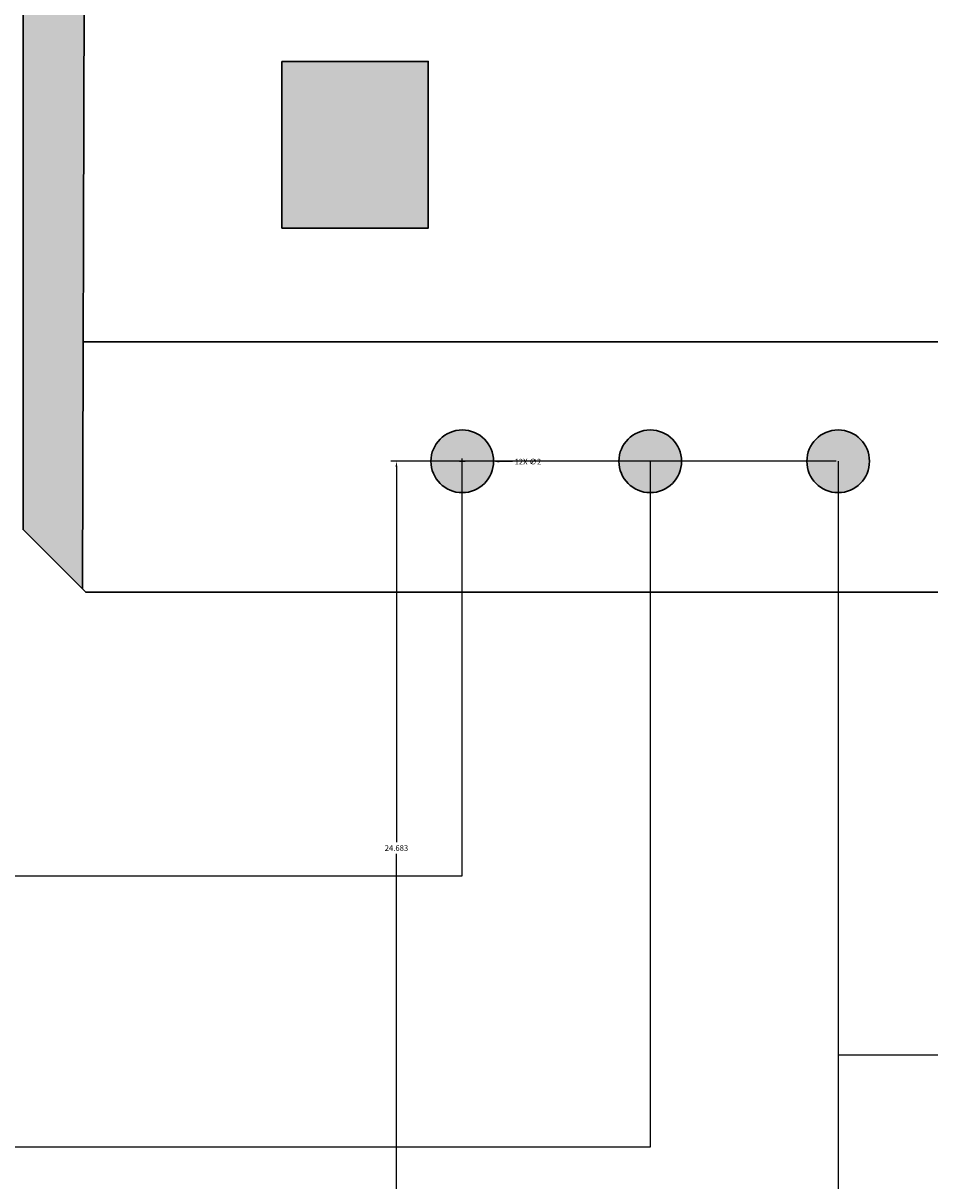
# Model space of a CAD drawing. Units: millimetres. Extents: x -8 to 285, y 5 to 221.
# Tile 5 of 30: x 26 to 55, y 45 to 82. Entities that reach past the tile are written whole.
import ezdxf

# ---------------------------------------------------------------- set-up
doc = ezdxf.new("R2010")
doc.units = ezdxf.units.MM
for name, color, linetype, lineweight in [('A-ANNO-DIMS', 2, 'Continuous', 18), ('E-EQPM-PATT', 252, 'Continuous', 13), ('E-POWR-CTRL', 7, 'Continuous', 30), ('E-POWR-DC-NEG', 3, 'Continuous', 25)]:
    doc.layers.add(name, color=color, linetype=linetype, lineweight=lineweight)
doc.layers.add('E-POWR-DC-POS', color=30, linetype='Continuous', lineweight=25, true_color=0xf26722)
doc.styles.get("Standard").update_dxf_attribs({"font": 'arial.ttf'})
doc.dimstyles.get("Standard").update_dxf_attribs({"dimtxt": 0.18, "dimasz": 0.18, "dimexe": 0.18, "dimexo": 0.0625, "dimgap": 0.09, "dimtad": 0, "dimtih": 1, "dimtoh": 1, "dimdec": 4, "dimzin": 0, "dimdsep": 46, "dimtxsty": 'Standard', "dimcen": 0.09, "dimadec": 0, "dimazin": 0, "dimtfac": 1, "dimtdec": 4, "dimtofl": 0, "dimtmove": 0, "dimatfit": 3, "dimfxl": 1, "dimtolj": 1, "dimtzin": 0, "dimarcsym": 0})

# ---------------------------------------------------------------- blocks, each defined once
blk = doc.blocks.new('*D10')
at = {"layer": 'A-ANNO-DIMS', "color": 0, "lineweight": -2, "transparency": 16777216}
for p, q in [((145.103, 206.457), (-7.608, 206.457)), ((-7.428, 206.277), (-7.428, 113.161)), ((-7.428, 19.682), (-7.428, 112.797)), ((30.453, 19.502), (-7.608, 19.502))]:
    blk.add_line(p, q, dxfattribs=at)
at = {"layer": 'A-ANNO-DIMS', "color": 0, "transparency": 16777216}
for points in [[(-7.458, 206.277), (-7.398, 206.277), (-7.428, 206.457)], [(-7.458, 19.682), (-7.398, 19.682), (-7.428, 19.502)]]:
    blk.add_solid(points, dxfattribs=at)
at = {"layer": 'Defpoints', "color": 0, "transparency": 16777216}
for p in [(-7.428, 206.457), (145.165, 206.457), (30.516, 19.502)]:
    blk.add_point(p, dxfattribs=at)
at = {"layer": 'A-ANNO-DIMS', "color": 0, "transparency": 16777216, "insert": (-7.428, 112.979), "char_height": 0.18, "attachment_point": 5}
blk.add_mtext('\\A1;186.95', dxfattribs=at)
blk = doc.blocks.new('*D21')
at = {"layer": 'A-ANNO-DIMS', "color": 0, "lineweight": -2, "transparency": 16777216}
for p, q in [((52.109, 67.906), (37.892, 67.906)), ((38.072, 67.726), (38.072, 55.747)), ((38.072, 43.404), (38.072, 55.383)), ((52.109, 43.224), (37.892, 43.224))]:
    blk.add_line(p, q, dxfattribs=at)
at = {"layer": 'A-ANNO-DIMS', "color": 0, "transparency": 16777216}
for points in [[(38.042, 67.726), (38.102, 67.726), (38.072, 67.906)], [(38.042, 43.404), (38.102, 43.404), (38.072, 43.224)]]:
    blk.add_solid(points, dxfattribs=at)
at = {"layer": 'Defpoints', "color": 0, "transparency": 16777216}
for p in [(38.072, 67.906), (52.172, 67.906), (52.172, 43.224)]:
    blk.add_point(p, dxfattribs=at)
at = {"layer": 'A-ANNO-DIMS', "color": 0, "transparency": 16777216, "insert": (38.072, 55.565), "char_height": 0.18, "attachment_point": 5}
blk.add_mtext('\\A1;24.683', dxfattribs=at)
blk = doc.blocks.new('*D22')
at = {"layer": 'A-ANNO-DIMS', "color": 0, "lineweight": -2, "transparency": 16777216}
for p, q in [((6.672, 45.959), (6.672, 5.222)), ((30.516, 35.867), (30.516, 5.222)), ((6.852, 5.402), (18.129, 5.402)), ((30.336, 5.402), (19.059, 5.402))]:
    blk.add_line(p, q, dxfattribs=at)
at = {"layer": 'A-ANNO-DIMS', "color": 0, "transparency": 16777216}
for points in [[(6.852, 5.432), (6.852, 5.372), (6.672, 5.402)], [(30.336, 5.432), (30.336, 5.372), (30.516, 5.402)]]:
    blk.add_solid(points, dxfattribs=at)
at = {"layer": 'Defpoints', "color": 0, "transparency": 16777216}
for p in [(6.672, 46.021), (30.516, 35.929), (30.516, 5.402)]:
    blk.add_point(p, dxfattribs=at)
at = {"layer": 'A-ANNO-DIMS', "color": 0, "transparency": 16777216, "insert": (18.594, 5.402), "char_height": 0.18, "attachment_point": 5}
blk.add_mtext('\\A1;23.843', dxfattribs=at)
blk = doc.blocks.new('*D38')
at = {"layer": 'A-ANNO-DIMS', "color": 0, "lineweight": -2, "transparency": 16777216}
for p, q in [((40.172, 67.816), (40.172, 67.996)), ((40.082, 67.906), (40.262, 67.906)), ((41.772, 67.896), (41.352, 67.899))]:
    blk.add_line(p, q, dxfattribs=at)
at = {"layer": 'A-ANNO-DIMS', "color": 0, "transparency": 16777216}
blk.add_solid([(41.352, 67.929), (41.351, 67.869), (41.172, 67.9)], dxfattribs=at)
at = {"layer": 'Defpoints', "color": 0, "transparency": 16777216}
for p in [(39.172, 67.913), (41.172, 67.9)]:
    blk.add_point(p, dxfattribs=at)
at = {"layer": 'A-ANNO-DIMS', "color": 0, "transparency": 16777216, "insert": (42.268, 67.896), "char_height": 0.18, "attachment_point": 5}
blk.add_mtext('\\A1;12X ∅2', dxfattribs=at)

msp = doc.modelspace()

# ---------------------------------------------------------------- hatches: boundary and pattern name
at = {"layer": 'E-EQPM-PATT'}
h = msp.add_hatch(color=256, dxfattribs=at)
h.set_gradient(color2=(0, 0, 0), tint=1)
h.paths.add_polyline_path([(41.1717, 67.9064, 1), (39.1717, 67.9064, 1)])
h.paths.add_polyline_path([(47.1717, 67.9064, 1), (45.1717, 67.9064, 1)])
h.paths.add_polyline_path([(53.1717, 67.9064, 1), (51.1717, 67.9064, 1)])
h.paths.add_polyline_path([(57.1717, 67.9064, 1), (59.1717, 67.9064, 1)])
h.paths.add_polyline_path([(65.1717, 67.9064, 1), (63.1717, 67.9064, 1)])
h.paths.add_polyline_path([(69.1717, 67.9064, 1), (71.1717, 67.9064, 1)])
h.paths.add_polyline_path([(148.1394, 196.6424), (148.1394, 201.7939), (142.1909, 201.7939), (142.1909, 196.6424)])
h.paths.add_polyline_path([(186.1388, 201.7939), (186.1388, 196.6424), (192.0873, 196.6424), (192.0873, 201.7939)])
h.paths.add_polyline_path([(234.0155, 196.6424), (234.0155, 201.7939), (228.067, 201.7939), (228.067, 196.6424)])
h = msp.add_hatch(color=256, dxfattribs=at)
h.set_gradient(color1=(248, 153, 30), color2=(248, 153, 30), tint=1)
h.paths.add_polyline_path([(28.1554, 99.1437), (26.1554, 97.1437), (26.1554, 65.7282), (28.0483, 63.8353)])
h.paths.add_polyline_path([(81.859, 63.7282), (83.859, 65.7282), (83.859, 97.1437), (81.859, 99.1437)])
h.paths.add_polyline_path([(39.086, 92.2191), (34.4177, 92.2191), (34.4177, 86.904), (39.086, 86.904)])
h.paths.add_polyline_path([(74.424, 86.904), (74.424, 92.2191), (69.7557, 92.2191), (69.7557, 86.904)])
h.paths.add_polyline_path([(74.5326, 81.2093), (69.8643, 81.2093), (69.8643, 75.8943), (74.5326, 75.8943)])
h.paths.add_polyline_path([(34.4177, 75.3519), (39.086, 75.3519), (39.086, 80.667), (34.4177, 80.667)])

# ---------------------------------------------------------------- linework, layer by layer
at = {"layer": 'E-POWR-CTRL'}
for p, q in [((28.1554, 99.1437), (28.0483, 63.8353)), ((28.0722, 71.7183), (81.859, 71.7183))]:
    msp.add_line(p, q, dxfattribs=at)
for points in [[(28.1554, 99.1437), (81.859, 99.1437), (83.859, 97.1437), (83.859, 65.7282), (81.859, 63.7282), (28.1554, 63.7282), (26.1554, 65.7282), (26.1554, 97.1437)], [(34.4177, 80.667), (39.086, 80.667), (39.086, 75.3519), (34.4177, 75.3519)]]:
    msp.add_lwpolyline(points, close=True, dxfattribs=at)
for centre in [(40.1717, 67.9064), (46.1717, 67.9064), (52.1717, 67.9064)]:
    msp.add_circle(centre, 1, dxfattribs=at)
at = {"layer": 'E-POWR-DC-NEG'}
msp.add_lwpolyline([(46.1717, 67.9064), (46.1717, 46.0211), (6.6725, 46.0211), (6.6725, 133.7273), (20.0566, 133.7273), (20.0566, 145.2715)], dxfattribs=at)
at = {"layer": 'E-POWR-DC-POS'}
for points in [[(74.9801, 145.2715), (74.9801, 123.1618), (17.279, 123.1618), (17.279, 54.6776), (40.1717, 54.6776), (40.1717, 67.9064)], [(52.1717, 67.9064), (52.1717, 43.2239), (38.1745, 43.2239), (38.1745, 38.4537)], [(52.1717, 48.962), (202.4345, 48.962), (202.4345, 34.9746)]]:
    msp.add_lwpolyline(points, dxfattribs=at)

# ---------------------------------------------------------------- dimensions: what is measured, and where the dimension line sits
at = {"layer": 'A-ANNO-DIMS'}
for base, p1, p2, override, picture, middle in [((-7.4275, 206.4568), (30.516, 19.502), (145.1651, 206.4568), {"dimdec": 2, "dimlfac": 1, "dimrnd": 0, "dimzin": 0, "dimdsep": 46, "dimlunit": 2}, '*D10', (-7.4275, 112.9794)), ((38.07166, 67.90641), (52.17166, 43.22389), (52.17166, 67.90641), {"dimdec": 3, "dimlfac": 1, "dimrnd": 0, "dimzin": 0, "dimdsep": 46, "dimlunit": 2}, '*D21', (38.07166, 55.56515))]:
    dim = msp.add_linear_dim(base=base, p1=p1, p2=p2, angle=90, dimstyle='Standard', override=override, dxfattribs=at)
    dim.commit()
    dim.dimension.update_dxf_attribs({"geometry": picture, "text_midpoint": middle})
dim = msp.add_diameter_dim_2p(p1=(39.1717, 67.913), p2=(41.1716, 67.8999), text='12X <>', dimstyle='Standard', override={"dimdec": 0, "dimlfac": 1, "dimrnd": 0, "dimzin": 0, "dimdsep": 46, "dimlunit": 2}, dxfattribs=at)
dim.commit()
dim.dimension.update_dxf_attribs({"geometry": '*D38', "text_midpoint": (41.7716, 67.8959), "dimtype": 163})
dim = msp.add_linear_dim(base=(30.51597, 5.40199), p1=(6.67248, 46.02115), p2=(30.51597, 35.92922), dimstyle='Standard', override={"dimdec": 3, "dimlfac": 1, "dimrnd": 0, "dimzin": 0, "dimdsep": 46, "dimlunit": 2}, dxfattribs=at)
dim.commit()
dim.dimension.update_dxf_attribs({"geometry": '*D22', "text_midpoint": (18.59423, 5.40199)})

doc.saveas('drawing.dxf')
